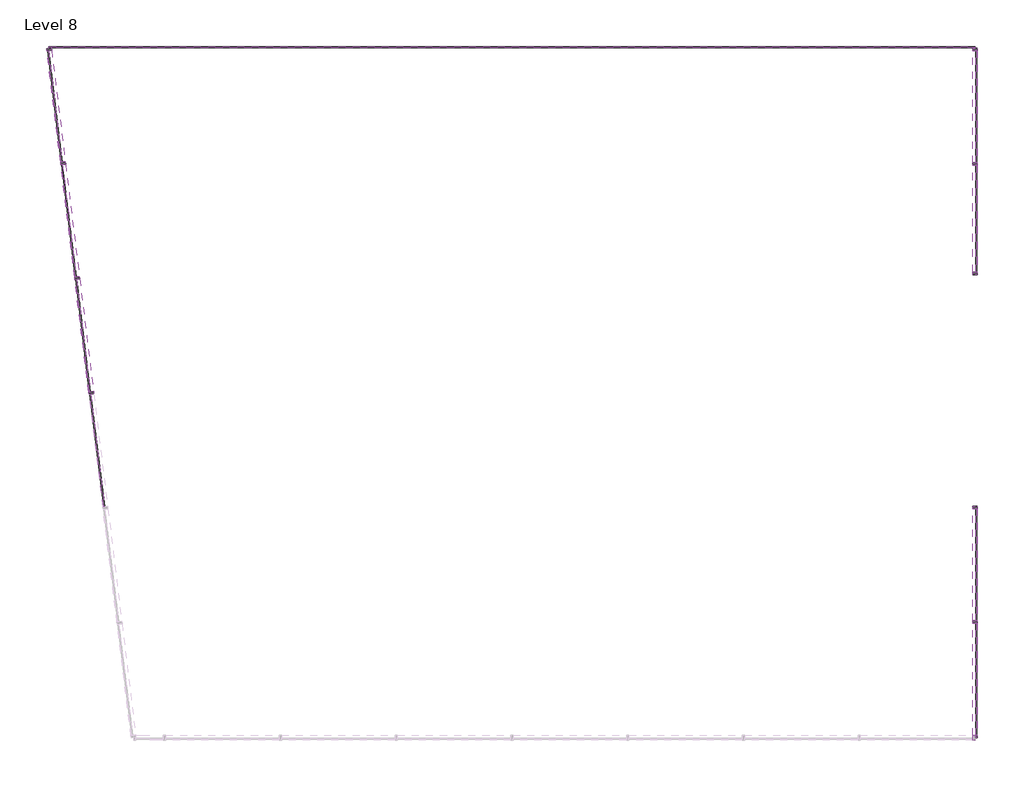
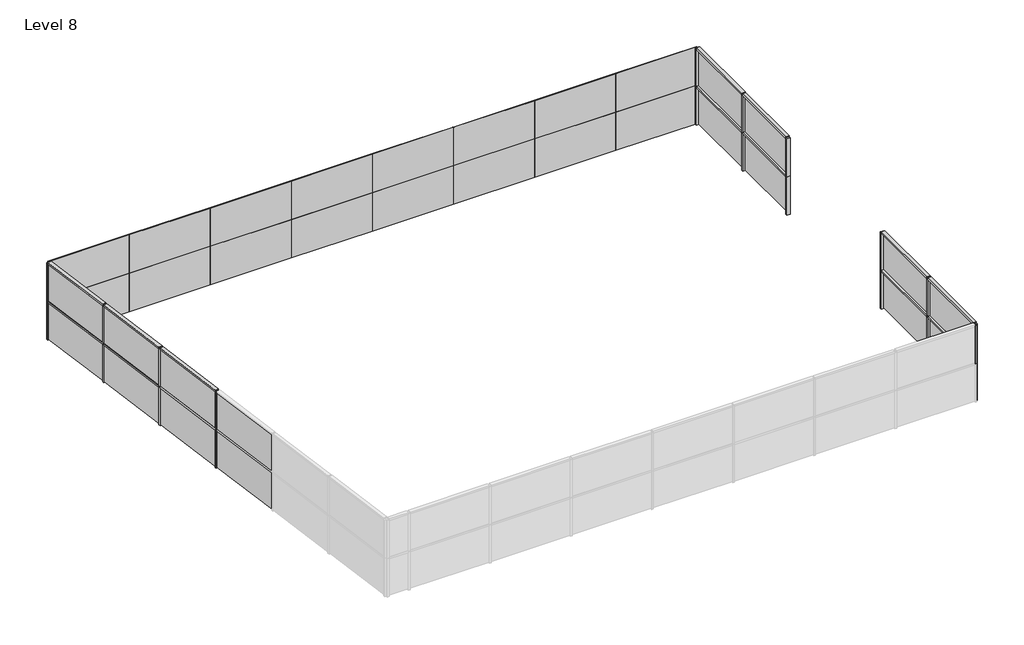
# One storey, part 2 of 2: 35 members, 32 plates.
"""IFC4 building model written with IfcOpenShell, lengths in millimetres."""

from ifc_helpers import new_model, si_unit, origin, place, context, project, spatial, transform, mapped, element, save
from components import member_19d0a4ec, member_8cef0660, member_82905deb, member_4491d118, member_46bdb8c2, system_panel_glazed_1e57f9bb, system_panel_glazed_e46d4b42, system_panel_glazed_2a6c68b7, system_panel_glazed_d483336f

model = new_model("IFC4")

# Units and contexts
model_context = context("Model", 3, world=origin())
ifc_project = project(units=[si_unit("LENGTHUNIT", "METRE", prefix="MILLI")], contexts=[model_context])

# Site, building, storey
site = spatial("IfcSite", under=ifc_project)
building = spatial("IfcBuilding", under=site)
storey = spatial("IfcBuildingStorey", under=building, Name="Level 8", Elevation=21336.0)

# Members
placement = place(None, origin())
member_shape = member_19d0a4ec(model_context)
element("IfcMember", 1, ObjectType="Rectangular Mullion : 2.5\" x 5\" rectangular", at=placement, inside=storey, context=model_context, shape_type="MappedRepresentation", body=[
    mapped(member_shape, transform((-10113.8959567, 8178.7803212, 22860.0), x_axis=(0.0, 0.0, 1.0), y_axis=(-0.9925461516413222, -0.12186934340514599, 0.0), z_axis=(0.12186934340514599, -0.9925461516413222, 0.0))),
])
element("IfcMember", 2, ObjectType="Rectangular Mullion : 2.5\" x 5\" rectangular", at=placement, inside=storey, context=model_context, shape_type="MappedRepresentation", body=[
    mapped(member_shape, transform((-10113.8959567, 8178.7803212, 24384.0), x_axis=(0.0, 0.0, 1.0), y_axis=(-0.9925461516413222, -0.12186934340514599, 0.0), z_axis=(0.12186934340514599, -0.9925461516413222, 0.0))),
])
element("IfcMember", 3, ObjectType="Rectangular Mullion : 2.5\" x 5\" rectangular", at=placement, inside=storey, context=model_context, shape_type="MappedRepresentation", body=[
    mapped(member_shape, transform((13902.5156363, -946.6363705, 22860.0), x_axis=(0.0, 0.0, 1.0), y_axis=(1.0, 0.0, 0.0), z_axis=(0.0, 1.0, 0.0))),
])
element("IfcMember", 4, ObjectType="Rectangular Mullion : 2.5\" x 5\" rectangular", at=placement, inside=storey, context=model_context, shape_type="MappedRepresentation", body=[
    mapped(member_shape, transform((13902.5156363, -3962.8863708, 22860.0), x_axis=(0.0, 0.0, 1.0), y_axis=(1.0, 0.0, 0.0), z_axis=(0.0, 1.0, 0.0))),
])
element("IfcMember", 5, ObjectType="Rectangular Mullion : 2.5\" x 5\" rectangular", at=placement, inside=storey, context=model_context, shape_type="MappedRepresentation", body=[
    mapped(member_shape, transform((13902.5156363, -946.6363705, 24384.0), x_axis=(0.0, 0.0, 1.0), y_axis=(1.0, 0.0, 0.0), z_axis=(0.0, 1.0, 0.0))),
])
element("IfcMember", 6, ObjectType="Rectangular Mullion : 2.5\" x 5\" rectangular", at=placement, inside=storey, context=model_context, shape_type="MappedRepresentation", body=[
    mapped(member_shape, transform((13902.5156363, -3962.8863708, 24384.0), x_axis=(0.0, 0.0, 1.0), y_axis=(1.0, 0.0, 0.0), z_axis=(0.0, 1.0, 0.0))),
])
element("IfcMember", 7, ObjectType="Rectangular Mullion : 2.5\" x 5\" rectangular", at=placement, inside=storey, context=model_context, shape_type="MappedRepresentation", body=[
    mapped(member_shape, transform((13902.5156363, 11109.0476508, 22860.0), x_axis=(0.0, 0.0, 1.0), y_axis=(1.0, 0.0, 0.0), z_axis=(0.0, 1.0, 0.0))),
])
element("IfcMember", 8, ObjectType="Rectangular Mullion : 2.5\" x 5\" rectangular", at=placement, inside=storey, context=model_context, shape_type="MappedRepresentation", body=[
    mapped(member_shape, transform((13902.5156363, 11109.0476508, 24384.0), x_axis=(0.0, 0.0, 1.0), y_axis=(1.0, 0.0, 0.0), z_axis=(0.0, 1.0, 0.0))),
])
member_2_shape = member_8cef0660(model_context)
element("IfcMember", 9, ObjectType="Rectangular Mullion : 2.5\" x 5\" rectangular", at=placement, inside=storey, context=model_context, shape_type="MappedRepresentation", body=[
    mapped(member_2_shape, transform((-9370.9804393, 2128.2189808, 22860.0), x_axis=(0.0, 0.0, 1.0), y_axis=(-0.9925461516413223, -0.12186934340514562, 0.0), z_axis=(0.12186934340514562, -0.9925461516413223, 0.0))),
])
element("IfcMember", 10, ObjectType="Rectangular Mullion : 2.5\" x 5\" rectangular", at=placement, inside=storey, context=model_context, shape_type="MappedRepresentation", body=[
    mapped(member_2_shape, transform((-9742.438198, 5153.499651, 22860.0), x_axis=(0.0, 0.0, 1.0), y_axis=(-0.9925461516413222, -0.12186934340514606, 0.0), z_axis=(0.12186934340514606, -0.9925461516413222, 0.0))),
])
element("IfcMember", 11, ObjectType="Rectangular Mullion : 2.5\" x 5\" rectangular", at=placement, inside=storey, context=model_context, shape_type="MappedRepresentation", body=[
    mapped(member_2_shape, transform((-9370.9804393, 2128.2189808, 24384.0), x_axis=(0.0, 0.0, 1.0), y_axis=(-0.9925461516413222, -0.12186934340514595, 0.0), z_axis=(0.12186934340514595, -0.9925461516413222, 0.0))),
])
element("IfcMember", 12, ObjectType="Rectangular Mullion : 2.5\" x 5\" rectangular", at=placement, inside=storey, context=model_context, shape_type="MappedRepresentation", body=[
    mapped(member_2_shape, transform((-9742.438198, 5153.499651, 24384.0), x_axis=(0.0, 0.0, 1.0), y_axis=(-0.9925461516413222, -0.1218693434051457, 0.0), z_axis=(0.1218693434051457, -0.9925461516413222, 0.0))),
])
member_3_shape = member_82905deb(model_context)
element("IfcMember", 13, ObjectType="Rectangular Mullion : 2.5\" x 5\" rectangular", at=placement, inside=storey, context=model_context, shape_type="MappedRepresentation", body=[
    mapped(member_3_shape, transform((-9367.1110876, 2096.7056405, 22860.0), x_axis=(-0.1218693434051459, 0.9925461516413222, 0.0), y_axis=(-0.9925461516413222, -0.1218693434051459, 0.0), z_axis=(0.0, 0.0, 1.0))),
])
element("IfcMember", 14, ObjectType="Rectangular Mullion : 2.5\" x 5\" rectangular", at=placement, inside=storey, context=model_context, shape_type="MappedRepresentation", body=[
    mapped(member_3_shape, transform((-9367.1110876, 2096.7056405, 24384.0), x_axis=(-0.1218693434051459, 0.9925461516413222, 0.0), y_axis=(-0.9925461516413222, -0.1218693434051459, 0.0), z_axis=(0.0, 0.0, 1.0))),
])
element("IfcMember", 15, ObjectType="Rectangular Mullion : 2.5\" x 5\" rectangular", at=placement, inside=storey, context=model_context, shape_type="MappedRepresentation", body=[
    mapped(member_3_shape, transform((-9738.5688463, 5121.9863107, 22860.0), x_axis=(-0.1218693434051459, 0.9925461516413222, 0.0), y_axis=(-0.9925461516413222, -0.1218693434051459, 0.0), z_axis=(0.0, 0.0, 1.0))),
])
element("IfcMember", 16, ObjectType="Rectangular Mullion : 2.5\" x 5\" rectangular", at=placement, inside=storey, context=model_context, shape_type="MappedRepresentation", body=[
    mapped(member_3_shape, transform((-9738.5688463, 5121.9863107, 24384.0), x_axis=(-0.1218693434051459, 0.9925461516413222, 0.0), y_axis=(-0.9925461516413222, -0.1218693434051459, 0.0), z_axis=(0.0, 0.0, 1.0))),
])
element("IfcMember", 17, ObjectType="Rectangular Mullion : 2.5\" x 5\" rectangular", at=placement, inside=storey, context=model_context, shape_type="MappedRepresentation", body=[
    mapped(member_3_shape, transform((-10110.026605, 8147.2669809, 22860.0), x_axis=(-0.1218693434051459, 0.9925461516413222, 0.0), y_axis=(-0.9925461516413222, -0.1218693434051459, 0.0), z_axis=(0.0, 0.0, 1.0))),
])
element("IfcMember", 18, ObjectType="Rectangular Mullion : 2.5\" x 5\" rectangular", at=placement, inside=storey, context=model_context, shape_type="MappedRepresentation", body=[
    mapped(member_3_shape, transform((-10110.026605, 8147.2669809, 24384.0), x_axis=(-0.1218693434051459, 0.9925461516413222, 0.0), y_axis=(-0.9925461516413222, -0.1218693434051459, 0.0), z_axis=(0.0, 0.0, 1.0))),
])
element("IfcMember", 19, ObjectType="Rectangular Mullion : 2.5\" x 5\" rectangular", at=placement, inside=storey, context=model_context, shape_type="MappedRepresentation", body=[
    mapped(member_3_shape, transform((13902.5156363, -3931.1363708, 22860.0), x_axis=(0.0, -1.0, 0.0), y_axis=(1.0, 0.0, 0.0), z_axis=(0.0, 0.0, 1.0))),
])
element("IfcMember", 20, ObjectType="Rectangular Mullion : 2.5\" x 5\" rectangular", at=placement, inside=storey, context=model_context, shape_type="MappedRepresentation", body=[
    mapped(member_3_shape, transform((13902.5156363, -3931.1363708, 24384.0), x_axis=(0.0, -1.0, 0.0), y_axis=(1.0, 0.0, 0.0), z_axis=(0.0, 0.0, 1.0))),
])
element("IfcMember", 21, ObjectType="Rectangular Mullion : 2.5\" x 5\" rectangular", at=placement, inside=storey, context=model_context, shape_type="MappedRepresentation", body=[
    mapped(member_3_shape, transform((13902.5156363, 8124.5476505, 22860.0), x_axis=(0.0, -1.0, 0.0), y_axis=(1.0, 0.0, 0.0), z_axis=(0.0, 0.0, 1.0))),
])
element("IfcMember", 22, ObjectType="Rectangular Mullion : 2.5\" x 5\" rectangular", at=placement, inside=storey, context=model_context, shape_type="MappedRepresentation", body=[
    mapped(member_3_shape, transform((13902.5156363, 8124.5476505, 24384.0), x_axis=(0.0, -1.0, 0.0), y_axis=(1.0, 0.0, 0.0), z_axis=(0.0, 0.0, 1.0))),
])
member_4_shape = member_4491d118(model_context)
element("IfcMember", 23, ObjectType="Rectangular Mullion : 2.5\" x 5\" rectangular", at=placement, inside=storey, context=model_context, shape_type="MappedRepresentation", body=[
    mapped(member_4_shape, transform((13902.5156363, -6979.1363705, 22860.0), x_axis=(1.0, 0.0, 0.0), y_axis=(0.0, -1.0, 0.0), z_axis=(0.0, 0.0, -1.0))),
])
element("IfcMember", 24, ObjectType="Rectangular Mullion : 2.5\" x 5\" rectangular", at=placement, inside=storey, context=model_context, shape_type="MappedRepresentation", body=[
    mapped(member_4_shape, transform((13902.5156363, -883.1363705, 21336.0), x_axis=(0.0, 1.0, 0.0), y_axis=(1.0, 0.0, 0.0), z_axis=(0.0, 0.0, -1.0))),
])
element("IfcMember", 25, ObjectType="Rectangular Mullion : 2.5\" x 5\" rectangular", at=placement, inside=storey, context=model_context, shape_type="MappedRepresentation", body=[
    mapped(member_4_shape, transform((13902.5156363, -883.1363705, 22860.0), x_axis=(0.0, 1.0, 0.0), y_axis=(1.0, 0.0, 0.0), z_axis=(0.0, 0.0, -1.0))),
])
element("IfcMember", 26, ObjectType="Rectangular Mullion : 2.5\" x 5\" rectangular", at=placement, inside=storey, context=model_context, shape_type="MappedRepresentation", body=[
    mapped(member_4_shape, transform((13902.5156363, 11172.5476508, 21336.0), x_axis=(0.0, 1.0, 0.0), y_axis=(1.0, 0.0, 0.0), z_axis=(0.0, 0.0, -1.0))),
])
element("IfcMember", 27, ObjectType="Rectangular Mullion : 2.5\" x 5\" rectangular", at=placement, inside=storey, context=model_context, shape_type="MappedRepresentation", body=[
    mapped(member_4_shape, transform((13902.5156363, 11172.5476508, 22860.0), x_axis=(0.0, 1.0, 0.0), y_axis=(1.0, 0.0, 0.0), z_axis=(0.0, 0.0, -1.0))),
])
element("IfcMember", 28, ObjectType="Rectangular Mullion : 2.5\" x 5\" rectangular", at=placement, inside=storey, context=model_context, shape_type="MappedRepresentation", body=[
    mapped(member_4_shape, transform((-10481.4843637, 11172.5476508, 22860.0), x_axis=(-0.1218693434051459, 0.9925461516413222, 0.0), y_axis=(-0.9925461516413222, -0.1218693434051459, 0.0), z_axis=(0.0, 0.0, 1.0))),
])
element("IfcMember", 29, ObjectType="Rectangular Mullion : 2.5\" x 5\" rectangular", at=placement, inside=storey, context=model_context, shape_type="MappedRepresentation", body=[
    mapped(member_4_shape, transform((-10481.4843637, 11172.5476508, 24384.0), x_axis=(-0.1218693434051459, 0.9925461516413222, 0.0), y_axis=(-0.9925461516413222, -0.1218693434051459, 0.0), z_axis=(0.0, 0.0, 1.0))),
])
element("IfcMember", 30, ObjectType="Rectangular Mullion : 2.5\" x 5\" rectangular", at=placement, inside=storey, context=model_context, shape_type="MappedRepresentation", body=[
    mapped(member_4_shape, transform((13902.5156363, -6979.1363705, 22860.0), x_axis=(0.0, -1.0, 0.0), y_axis=(1.0, 0.0, 0.0), z_axis=(0.0, 0.0, 1.0))),
])
element("IfcMember", 31, ObjectType="Rectangular Mullion : 2.5\" x 5\" rectangular", at=placement, inside=storey, context=model_context, shape_type="MappedRepresentation", body=[
    mapped(member_4_shape, transform((13902.5156363, -6979.1363705, 24384.0), x_axis=(0.0, -1.0, 0.0), y_axis=(1.0, 0.0, 0.0), z_axis=(0.0, 0.0, 1.0))),
])
element("IfcMember", 32, ObjectType="Rectangular Mullion : 2.5\" x 5\" rectangular", at=placement, inside=storey, context=model_context, shape_type="MappedRepresentation", body=[
    mapped(member_4_shape, transform((13902.5156363, 5212.8636295, 22860.0), x_axis=(0.0, -1.0, 0.0), y_axis=(1.0, 0.0, 0.0), z_axis=(0.0, 0.0, 1.0))),
])
element("IfcMember", 33, ObjectType="Rectangular Mullion : 2.5\" x 5\" rectangular", at=placement, inside=storey, context=model_context, shape_type="MappedRepresentation", body=[
    mapped(member_4_shape, transform((13902.5156363, 5212.8636295, 24384.0), x_axis=(0.0, -1.0, 0.0), y_axis=(1.0, 0.0, 0.0), z_axis=(0.0, 0.0, 1.0))),
])
member_5_shape = member_46bdb8c2(model_context)
element("IfcMember", 34, ObjectType="Rectangular Mullion : 2.5\" x 5\" rectangular", at=placement, inside=storey, context=model_context, shape_type="MappedRepresentation", body=[
    mapped(member_5_shape, transform((13902.5156363, 8092.7976505, 22860.0), x_axis=(0.0, 0.0, 1.0), y_axis=(1.0, 0.0, 0.0), z_axis=(0.0, 1.0, 0.0))),
])
element("IfcMember", 35, ObjectType="Rectangular Mullion : 2.5\" x 5\" rectangular", at=placement, inside=storey, context=model_context, shape_type="MappedRepresentation", body=[
    mapped(member_5_shape, transform((13902.5156363, 8092.7976505, 24384.0), x_axis=(0.0, 0.0, 1.0), y_axis=(1.0, 0.0, 0.0), z_axis=(0.0, 1.0, 0.0))),
])

# Plates
system_panel_glazed_shape = system_panel_glazed_1e57f9bb(model_context)
element("IfcPlate", 36, ObjectType="System Panel : Glazed", at=placement, inside=storey, context=model_context, shape_type="MappedRepresentation", body=[
    mapped(system_panel_glazed_shape, transform((-8957.4843636, 11172.5476508, 21336.0), x_axis=(1.0, 0.0, 0.0), y_axis=(0.0, 1.0, 0.0), z_axis=(0.0, 0.0, 1.0))),
])
element("IfcPlate", 37, ObjectType="System Panel : Glazed", at=placement, inside=storey, context=model_context, shape_type="MappedRepresentation", body=[
    mapped(system_panel_glazed_shape, transform((-5909.4843634, 11172.5476508, 21336.0), x_axis=(1.0, 0.0, 0.0), y_axis=(0.0, 1.0, 0.0), z_axis=(0.0, 0.0, 1.0))),
])
element("IfcPlate", 38, ObjectType="System Panel : Glazed", at=placement, inside=storey, context=model_context, shape_type="MappedRepresentation", body=[
    mapped(system_panel_glazed_shape, transform((-2861.4843634, 11172.5476508, 21336.0), x_axis=(1.0, 0.0, 0.0), y_axis=(0.0, 1.0, 0.0), z_axis=(0.0, 0.0, 1.0))),
])
element("IfcPlate", 39, ObjectType="System Panel : Glazed", at=placement, inside=storey, context=model_context, shape_type="MappedRepresentation", body=[
    mapped(system_panel_glazed_shape, transform((186.5156366, 11172.5476508, 21336.0), x_axis=(1.0, 0.0, 0.0), y_axis=(0.0, 1.0, 0.0), z_axis=(0.0, 0.0, 1.0))),
])
element("IfcPlate", 40, ObjectType="System Panel : Glazed", at=placement, inside=storey, context=model_context, shape_type="MappedRepresentation", body=[
    mapped(system_panel_glazed_shape, transform((3234.5156366, 11172.5476508, 21336.0), x_axis=(1.0, 0.0, 0.0), y_axis=(0.0, 1.0, 0.0), z_axis=(0.0, 0.0, 1.0))),
])
element("IfcPlate", 41, ObjectType="System Panel : Glazed", at=placement, inside=storey, context=model_context, shape_type="MappedRepresentation", body=[
    mapped(system_panel_glazed_shape, transform((6282.5156366, 11172.5476508, 21336.0), x_axis=(1.0, 0.0, 0.0), y_axis=(0.0, 1.0, 0.0), z_axis=(0.0, 0.0, 1.0))),
])
element("IfcPlate", 42, ObjectType="System Panel : Glazed", at=placement, inside=storey, context=model_context, shape_type="MappedRepresentation", body=[
    mapped(system_panel_glazed_shape, transform((9330.5156366, 11172.5476508, 21336.0), x_axis=(1.0, 0.0, 0.0), y_axis=(0.0, 1.0, 0.0), z_axis=(0.0, 0.0, 1.0))),
])
element("IfcPlate", 43, ObjectType="System Panel : Glazed", at=placement, inside=storey, context=model_context, shape_type="MappedRepresentation", body=[
    mapped(system_panel_glazed_shape, transform((12378.5156364, 11172.5476508, 21336.0), x_axis=(1.0, 0.0, 0.0), y_axis=(0.0, 1.0, 0.0), z_axis=(0.0, 0.0, 1.0))),
])
element("IfcPlate", 44, ObjectType="System Panel : Glazed", at=placement, inside=storey, context=model_context, shape_type="MappedRepresentation", body=[
    mapped(system_panel_glazed_shape, transform((-8957.4843636, 11172.5476508, 22860.0), x_axis=(1.0, 0.0, 0.0), y_axis=(0.0, 1.0, 0.0), z_axis=(0.0, 0.0, 1.0))),
])
element("IfcPlate", 45, ObjectType="System Panel : Glazed", at=placement, inside=storey, context=model_context, shape_type="MappedRepresentation", body=[
    mapped(system_panel_glazed_shape, transform((-5909.4843634, 11172.5476508, 22860.0), x_axis=(1.0, 0.0, 0.0), y_axis=(0.0, 1.0, 0.0), z_axis=(0.0, 0.0, 1.0))),
])
element("IfcPlate", 46, ObjectType="System Panel : Glazed", at=placement, inside=storey, context=model_context, shape_type="MappedRepresentation", body=[
    mapped(system_panel_glazed_shape, transform((-2861.4843634, 11172.5476508, 22860.0), x_axis=(1.0, 0.0, 0.0), y_axis=(0.0, 1.0, 0.0), z_axis=(0.0, 0.0, 1.0))),
])
element("IfcPlate", 47, ObjectType="System Panel : Glazed", at=placement, inside=storey, context=model_context, shape_type="MappedRepresentation", body=[
    mapped(system_panel_glazed_shape, transform((186.5156366, 11172.5476508, 22860.0), x_axis=(1.0, 0.0, 0.0), y_axis=(0.0, 1.0, 0.0), z_axis=(0.0, 0.0, 1.0))),
])
element("IfcPlate", 48, ObjectType="System Panel : Glazed", at=placement, inside=storey, context=model_context, shape_type="MappedRepresentation", body=[
    mapped(system_panel_glazed_shape, transform((3234.5156366, 11172.5476508, 22860.0), x_axis=(1.0, 0.0, 0.0), y_axis=(0.0, 1.0, 0.0), z_axis=(0.0, 0.0, 1.0))),
])
element("IfcPlate", 49, ObjectType="System Panel : Glazed", at=placement, inside=storey, context=model_context, shape_type="MappedRepresentation", body=[
    mapped(system_panel_glazed_shape, transform((6282.5156366, 11172.5476508, 22860.0), x_axis=(1.0, 0.0, 0.0), y_axis=(0.0, 1.0, 0.0), z_axis=(0.0, 0.0, 1.0))),
])
element("IfcPlate", 50, ObjectType="System Panel : Glazed", at=placement, inside=storey, context=model_context, shape_type="MappedRepresentation", body=[
    mapped(system_panel_glazed_shape, transform((9330.5156366, 11172.5476508, 22860.0), x_axis=(1.0, 0.0, 0.0), y_axis=(0.0, 1.0, 0.0), z_axis=(0.0, 0.0, 1.0))),
])
element("IfcPlate", 51, ObjectType="System Panel : Glazed", at=placement, inside=storey, context=model_context, shape_type="MappedRepresentation", body=[
    mapped(system_panel_glazed_shape, transform((12378.5156364, 11172.5476508, 22860.0), x_axis=(1.0, 0.0, 0.0), y_axis=(0.0, 1.0, 0.0), z_axis=(0.0, 0.0, 1.0))),
])
system_panel_glazed_2_shape = system_panel_glazed_e46d4b42(model_context)
element("IfcPlate", 52, ObjectType="System Panel : Glazed", at=placement, inside=storey, context=model_context, shape_type="MappedRepresentation", body=[
    mapped(system_panel_glazed_2_shape, transform((-10293.8208085, 9644.1506457, 21367.75), x_axis=(-0.1218693434051459, 0.9925461516413222, 0.0), y_axis=(-0.9925461516413222, -0.1218693434051459, 0.0), z_axis=(0.0, 0.0, 1.0))),
])
element("IfcPlate", 53, ObjectType="System Panel : Glazed", at=placement, inside=storey, context=model_context, shape_type="MappedRepresentation", body=[
    mapped(system_panel_glazed_2_shape, transform((-10293.8208085, 9644.1506457, 22891.75), x_axis=(-0.1218693434051459, 0.9925461516413222, 0.0), y_axis=(-0.9925461516413222, -0.1218693434051459, 0.0), z_axis=(0.0, 0.0, 1.0))),
])
element("IfcPlate", 54, ObjectType="System Panel : Glazed", at=placement, inside=storey, context=model_context, shape_type="MappedRepresentation", body=[
    mapped(system_panel_glazed_2_shape, transform((13902.5156363, -2423.0113706, 21367.75), x_axis=(0.0, -1.0, 0.0), y_axis=(1.0, 0.0, 0.0), z_axis=(0.0, 0.0, 1.0))),
])
element("IfcPlate", 55, ObjectType="System Panel : Glazed", at=placement, inside=storey, context=model_context, shape_type="MappedRepresentation", body=[
    mapped(system_panel_glazed_2_shape, transform((13902.5156363, -5439.2613706, 21367.75), x_axis=(0.0, -1.0, 0.0), y_axis=(1.0, 0.0, 0.0), z_axis=(0.0, 0.0, 1.0))),
])
element("IfcPlate", 56, ObjectType="System Panel : Glazed", at=placement, inside=storey, context=model_context, shape_type="MappedRepresentation", body=[
    mapped(system_panel_glazed_2_shape, transform((13902.5156363, -2423.0113706, 22891.75), x_axis=(0.0, -1.0, 0.0), y_axis=(1.0, 0.0, 0.0), z_axis=(0.0, 0.0, 1.0))),
])
element("IfcPlate", 57, ObjectType="System Panel : Glazed", at=placement, inside=storey, context=model_context, shape_type="MappedRepresentation", body=[
    mapped(system_panel_glazed_2_shape, transform((13902.5156363, -5439.2613706, 22891.75), x_axis=(0.0, -1.0, 0.0), y_axis=(1.0, 0.0, 0.0), z_axis=(0.0, 0.0, 1.0))),
])
element("IfcPlate", 58, ObjectType="System Panel : Glazed", at=placement, inside=storey, context=model_context, shape_type="MappedRepresentation", body=[
    mapped(system_panel_glazed_2_shape, transform((13902.5156363, 9632.6726506, 21367.75), x_axis=(0.0, -1.0, 0.0), y_axis=(1.0, 0.0, 0.0), z_axis=(0.0, 0.0, 1.0))),
])
element("IfcPlate", 59, ObjectType="System Panel : Glazed", at=placement, inside=storey, context=model_context, shape_type="MappedRepresentation", body=[
    mapped(system_panel_glazed_2_shape, transform((13902.5156363, 9632.6726506, 22891.75), x_axis=(0.0, -1.0, 0.0), y_axis=(1.0, 0.0, 0.0), z_axis=(0.0, 0.0, 1.0))),
])
system_panel_glazed_3_shape = system_panel_glazed_2a6c68b7(model_context)
element("IfcPlate", 60, ObjectType="System Panel : Glazed", at=placement, inside=storey, context=model_context, shape_type="MappedRepresentation", body=[
    mapped(system_panel_glazed_3_shape, transform((-9181.3822083, 584.0653054, 21367.75), x_axis=(-0.1218693434051459, 0.9925461516413222, 0.0), y_axis=(-0.9925461516413222, -0.1218693434051459, 0.0), z_axis=(0.0, 0.0, 1.0))),
])
element("IfcPlate", 61, ObjectType="System Panel : Glazed", at=placement, inside=storey, context=model_context, shape_type="MappedRepresentation", body=[
    mapped(system_panel_glazed_3_shape, transform((-9552.839967, 3609.3459756, 21367.75), x_axis=(-0.1218693434051459, 0.9925461516413222, 0.0), y_axis=(-0.9925461516413222, -0.1218693434051459, 0.0), z_axis=(0.0, 0.0, 1.0))),
])
element("IfcPlate", 62, ObjectType="System Panel : Glazed", at=placement, inside=storey, context=model_context, shape_type="MappedRepresentation", body=[
    mapped(system_panel_glazed_3_shape, transform((-9924.2977257, 6634.6266458, 21367.75), x_axis=(-0.1218693434051459, 0.9925461516413222, 0.0), y_axis=(-0.9925461516413222, -0.1218693434051459, 0.0), z_axis=(0.0, 0.0, 1.0))),
])
element("IfcPlate", 63, ObjectType="System Panel : Glazed", at=placement, inside=storey, context=model_context, shape_type="MappedRepresentation", body=[
    mapped(system_panel_glazed_3_shape, transform((-9181.3822083, 584.0653054, 22891.75), x_axis=(-0.1218693434051459, 0.9925461516413222, 0.0), y_axis=(-0.9925461516413222, -0.1218693434051459, 0.0), z_axis=(0.0, 0.0, 1.0))),
])
element("IfcPlate", 64, ObjectType="System Panel : Glazed", at=placement, inside=storey, context=model_context, shape_type="MappedRepresentation", body=[
    mapped(system_panel_glazed_3_shape, transform((-9552.839967, 3609.3459756, 22891.75), x_axis=(-0.1218693434051459, 0.9925461516413222, 0.0), y_axis=(-0.9925461516413222, -0.1218693434051459, 0.0), z_axis=(0.0, 0.0, 1.0))),
])
element("IfcPlate", 65, ObjectType="System Panel : Glazed", at=placement, inside=storey, context=model_context, shape_type="MappedRepresentation", body=[
    mapped(system_panel_glazed_3_shape, transform((-9924.2977257, 6634.6266458, 22891.75), x_axis=(-0.1218693434051459, 0.9925461516413222, 0.0), y_axis=(-0.9925461516413222, -0.1218693434051459, 0.0), z_axis=(0.0, 0.0, 1.0))),
])
system_panel_glazed_4_shape = system_panel_glazed_d483336f(model_context)
element("IfcPlate", 66, ObjectType="System Panel : Glazed", at=placement, inside=storey, context=model_context, shape_type="MappedRepresentation", body=[
    mapped(system_panel_glazed_4_shape, transform((13902.5156363, 6684.58064, 21367.75), x_axis=(0.0, -1.0, 0.0), y_axis=(1.0, 0.0, 0.0), z_axis=(0.0, 0.0, 1.0))),
])
element("IfcPlate", 67, ObjectType="System Panel : Glazed", at=placement, inside=storey, context=model_context, shape_type="MappedRepresentation", body=[
    mapped(system_panel_glazed_4_shape, transform((13902.5156363, 6684.58064, 22891.75), x_axis=(0.0, -1.0, 0.0), y_axis=(1.0, 0.0, 0.0), z_axis=(0.0, 0.0, 1.0))),
])

save(model, "model.ifc")

# Revit data of these elements
# Type "Rectangular Mullion : 2.5\" x 5\" rectangular"
#   built-in parameter 1007304 = 0.416667 (stored number, unit not read)
#   built-in parameter 1007301 = 0.104167 (stored number, unit not read)
#   built-in parameter 1007300 = 0.104167 (stored number, unit not read)
# Type "System Panel : Glazed"
#   Construction Type Id = "GSP4R"
#   Analytic Construction = "1/8 in Pilkington single glazing"
#   Visual Light Transmittance = 0.9
#   Solar Heat Gain Coefficient = 0.86
#   Heat Transfer Coefficient (U) = 1.18115 BTU/(h·ft²·°F)
#   Define Thermal Properties by = 1
# Elements 1, 2, 3, 4, 5, 6, 7, 8, 9, 10, 11, 12, 13, 14, 15, 16, 17, 18, 19, 20, 21, 22, 23, 24, 25, 26, 27, 28, 29, 30, 31, 32, 33, 34, 35 (IfcMember, "Rectangular Mullion : 2.5\" x 5\" rectangular")
#   Phase Created = New Construction
#   Materials on its faces: "Aluminum"
# Elements 36, 37, 38, 39, 40, 41, 42, 43, 44, 45, 46, 47, 48, 49, 50, 51, 52, 53, 54, 55, 56, 57, 58, 59, 60, 61, 62, 63, 64, 65, 66, 67 (IfcPlate, "System Panel : Glazed")
#   Phase Created = New Construction
#   Materials on its faces: "Glass"
# Materials
#   "Aluminum": class "Metal", colour RGB 247 247 247, transparency 0, Description = "Aluminum 6061", Cost = 0
#   "Glass": class "Glass", colour RGB 0 128 192, transparency 0.75, Description = "Soda Lime Glass", Cost = 0
